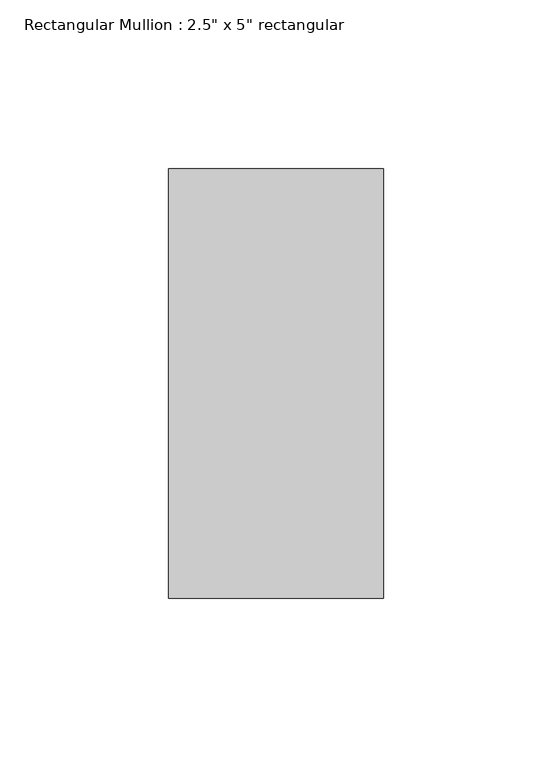
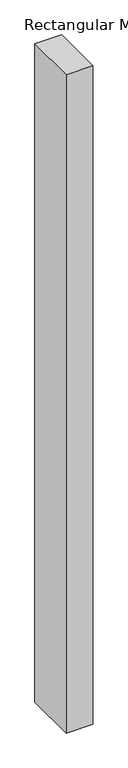
"""IFC4 building model written with IfcOpenShell, lengths in millimetres: member geometry."""

from ifc_helpers import new_model, si_unit, frame, origin, place, context, project, spatial, polyline, outline, extrude, source, transform, mapped, element, save


def member_067e20b4(model_context):
    return source(origin(), model_context, "Body", "SweptSolid", [
        extrude(outline(polyline([(0.0, 63.5), (0.0, -63.5), (-63.5, -63.5), (-63.5, 63.5), (0.0, 63.5)])), frame((0.0, 0.0, -1640.1839946), z_axis=(0.0, 0.0, 1.0), x_axis=(1.0, 0.0, 0.0)), (0.0, 0.0, 1.0), 1640.1839946),
    ])


if __name__ == "__main__":
    model = new_model("IFC4")
    model_context = context("Model", 3, world=origin())
    ifc_project = project(units=[si_unit("LENGTHUNIT", "METRE", prefix="MILLI")], contexts=[model_context])
    site = spatial("IfcSite", under=ifc_project)
    building = spatial("IfcBuilding", under=site)
    placement = place(None, origin())
    member_shape = member_067e20b4(model_context)
    element("IfcMember", 1, ObjectType="Rectangular Mullion : 2.5\" x 5\" rectangular", at=placement, inside=building, context=model_context, shape_type="MappedRepresentation", body=[
        mapped(member_shape, transform((0.0, 0.0, 0.0), x_axis=(1.0, 0.0, 0.0), y_axis=(0.0, 1.0, 0.0), z_axis=(0.0, 0.0, 1.0))),
    ])
    save(model, "model.ifc")

# Revit data of these elements
# Type "Rectangular Mullion : 2.5\" x 5\" rectangular"
#   built-in parameter 1007304 = 0.416667 (stored number, unit not read)
#   built-in parameter 1007301 = 0.104167 (stored number, unit not read)
#   built-in parameter 1007300 = 0.104167 (stored number, unit not read)
# Element 1 (IfcMember, "Rectangular Mullion : 2.5\" x 5\" rectangular")
#   Materials on its faces: "Aluminum"
# Materials
#   "Aluminum": class "Metal", colour RGB 247 247 247, transparency 0, Description = "Aluminum 6061", Cost = 0
